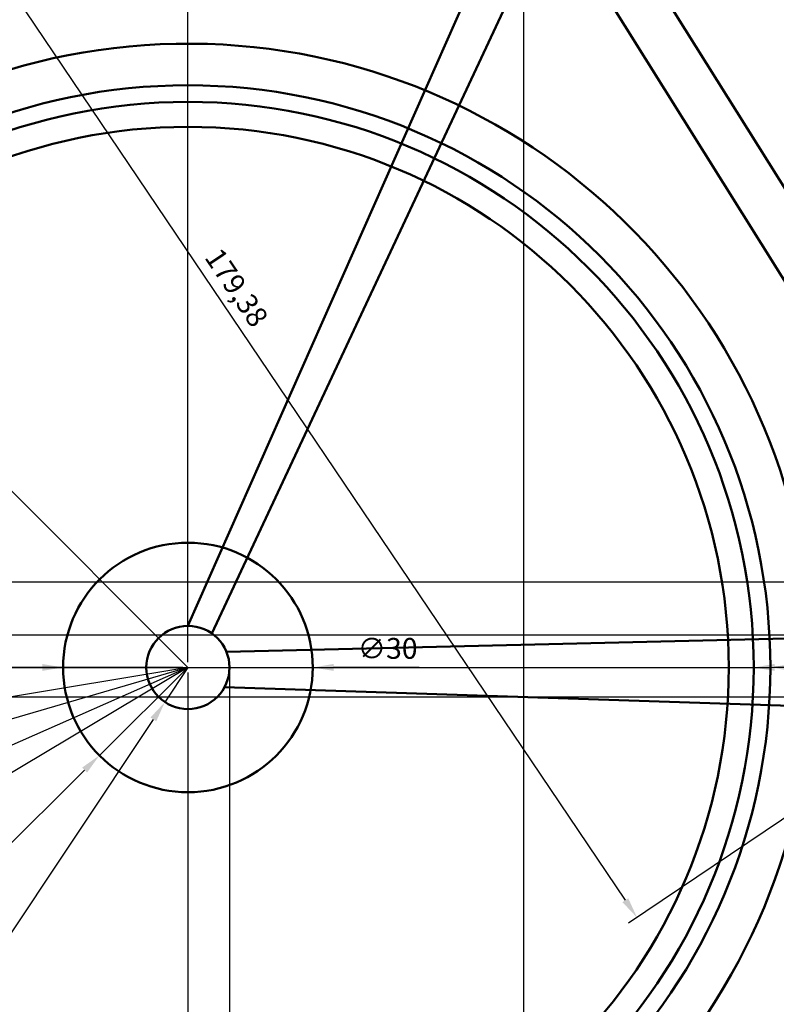
# Model space of a CAD drawing. Units: millimetres. Extents: x 1068 to 1546, y 1743 to 2032.
# Tile 3 of 9: x 1152 to 1243, y 1809 to 1928. Entities that reach past the tile are written whole.
import ezdxf

# ---------------------------------------------------------------- set-up
doc = ezdxf.new("R2010")
doc.units = ezdxf.units.MM
for name, color, linetype, lineweight in [('M-CONS', 8, 'Continuous', 18), ('M-DIMS', 2, 'Continuous', 25), ('M-OUTL', 7, 'Continuous', 50)]:
    doc.layers.add(name, color=color, linetype=linetype, lineweight=lineweight)
doc.styles.get("Standard").update_dxf_attribs({"font": 'arial.ttf'})
doc.dimstyles.new('ISO-25', dxfattribs={"dimtxt": 2.5, "dimasz": 2.5, "dimexe": 1.25, "dimexo": 0.625, "dimtad": 1, "dimtxsty": 'Standard', "dimcen": 2.5, "dimadec": 0, "dimazin": 0, "dimtfac": 1, "dimtmove": 0, "dimatfit": 3, "dimfxl": 1, "dimarcsym": 0})

# ---------------------------------------------------------------- blocks, each defined once
blk = doc.blocks.new('*D5')
at = {"layer": 'Defpoints', "color": 0, "transparency": 16777216}
for p in [(1177.23, 1849.76), (1402.23, 1849.76), (1402.23, 1747.98)]:
    blk.add_point(p, dxfattribs=at)
at = {"layer": 'M-DIMS', "color": 0, "lineweight": -2, "transparency": 16777216}
for p, q in [((1177.23, 1849.14), (1177.23, 1746.73)), ((1402.23, 1849.14), (1402.23, 1746.73)), ((1179.73, 1747.98), (1399.73, 1747.98))]:
    blk.add_line(p, q, dxfattribs=at)
at = {"layer": 'M-DIMS', "color": 0, "transparency": 16777216}
for points in [[(1179.73, 1748.39), (1179.73, 1747.56), (1177.23, 1747.98)], [(1399.73, 1748.39), (1399.73, 1747.56), (1402.23, 1747.98)]]:
    blk.add_solid(points, dxfattribs=at)
at = {"layer": 'M-DIMS', "color": 0, "transparency": 16777216, "insert": (1289.73, 1749.88), "char_height": 2.5, "attachment_point": 5}
blk.add_mtext('225', dxfattribs=at)
blk = doc.blocks.new('*D6')
at = {"layer": 'Defpoints', "color": 0, "transparency": 16777216}
for p in [(1172.23, 1849.76), (1270.79, 1849.76), (1270.79, 1762.16)]:
    blk.add_point(p, dxfattribs=at)
at = {"layer": 'M-DIMS', "color": 0, "lineweight": -2, "transparency": 16777216}
for p, q in [((1172.23, 1849.14), (1172.23, 1760.91)), ((1270.79, 1849.14), (1270.79, 1760.91)), ((1174.73, 1762.16), (1268.29, 1762.16))]:
    blk.add_line(p, q, dxfattribs=at)
at = {"layer": 'M-DIMS', "color": 0, "transparency": 16777216}
for points in [[(1174.73, 1762.57), (1174.73, 1761.74), (1172.23, 1762.16)], [(1268.29, 1762.57), (1268.29, 1761.74), (1270.79, 1762.16)]]:
    blk.add_solid(points, dxfattribs=at)
at = {"layer": 'M-DIMS', "color": 0, "transparency": 16777216, "insert": (1221.51, 1764.28), "char_height": 2.5, "attachment_point": 5}
blk.add_mtext('98,56', dxfattribs=at)
blk = doc.blocks.new('*D12')
at = {"layer": 'Defpoints', "color": 0, "transparency": 16777216}
for p in [(1172.23, 1849.76), (1169.46, 1845.6)]:
    blk.add_point(p, dxfattribs=at)
at = {"layer": 'M-DIMS', "color": 0, "lineweight": -2, "transparency": 16777216}
for p, q in [((1172.23, 1849.76), (1169.46, 1845.6)), ((1115.28, 1764.16), (1168.07, 1843.52))]:
    blk.add_line(p, q, dxfattribs=at)
at = {"layer": 'M-DIMS', "color": 0, "transparency": 16777216}
blk.add_solid([(1167.73, 1843.75), (1168.42, 1843.29), (1169.46, 1845.6)], dxfattribs=at)
at = {"layer": 'M-DIMS', "color": 0, "transparency": 16777216, "insert": (1115.17, 1767.42), "char_height": 2.5, "attachment_point": 5, "rotation": 56.3651}
blk.add_mtext('R5', dxfattribs=at)
blk = doc.blocks.new('*D13')
at = {"layer": 'Defpoints', "color": 0, "transparency": 16777216}
for p in [(1172.23, 1849.76), (1161.59, 1839.19)]:
    blk.add_point(p, dxfattribs=at)
at = {"layer": 'M-DIMS', "color": 0, "lineweight": -2, "transparency": 16777216}
for p, q in [((1172.23, 1849.76), (1161.59, 1839.19)), ((1102.29, 1780.3), (1159.81, 1837.43))]:
    blk.add_line(p, q, dxfattribs=at)
at = {"layer": 'M-DIMS', "color": 0, "transparency": 16777216}
blk.add_solid([(1159.52, 1837.73), (1160.11, 1837.13), (1161.59, 1839.19)], dxfattribs=at)
at = {"layer": 'M-DIMS', "color": 0, "transparency": 16777216, "insert": (1103.52, 1784.2), "char_height": 2.5, "attachment_point": 5, "rotation": 44.8055}
blk.add_mtext('R15', dxfattribs=at)
blk = doc.blocks.new('*D14')
at = {"layer": 'Defpoints', "color": 0, "transparency": 16777216}
for p in [(1172.23, 1849.76), (1116.4, 1816.48)]:
    blk.add_point(p, dxfattribs=at)
at = {"layer": 'M-DIMS', "color": 0, "lineweight": -2, "transparency": 16777216}
for p, q in [((1172.23, 1849.76), (1116.4, 1816.48)), ((1080.65, 1795.17), (1114.25, 1815.2))]:
    blk.add_line(p, q, dxfattribs=at)
at = {"layer": 'M-DIMS', "color": 0, "transparency": 16777216}
blk.add_solid([(1114.03, 1815.56), (1114.46, 1814.84), (1116.4, 1816.48)], dxfattribs=at)
at = {"layer": 'M-DIMS', "color": 0, "transparency": 16777216, "insert": (1082.79, 1798.66), "char_height": 2.5, "attachment_point": 5, "rotation": 30.7992}
blk.add_mtext('R65', dxfattribs=at)
blk = doc.blocks.new('*D15')
at = {"layer": 'Defpoints', "color": 0, "transparency": 16777216}
for p in [(1172.23, 1849.76), (1110.01, 1822.32)]:
    blk.add_point(p, dxfattribs=at)
at = {"layer": 'M-DIMS', "color": 0, "lineweight": -2, "transparency": 16777216}
for p, q in [((1172.23, 1849.76), (1110.01, 1822.32)), ((1084.58, 1811.1), (1107.72, 1821.31))]:
    blk.add_line(p, q, dxfattribs=at)
at = {"layer": 'M-DIMS', "color": 0, "transparency": 16777216}
blk.add_solid([(1107.55, 1821.69), (1107.89, 1820.93), (1110.01, 1822.32)], dxfattribs=at)
at = {"layer": 'M-DIMS', "color": 0, "transparency": 16777216, "insert": (1087.12, 1814.3), "char_height": 2.5, "attachment_point": 5, "rotation": 23.7993}
blk.add_mtext('R68', dxfattribs=at)
blk = doc.blocks.new('*D16')
at = {"layer": 'Defpoints', "color": 0, "transparency": 16777216}
for p in [(1172.23, 1849.76), (1105.05, 1830.07)]:
    blk.add_point(p, dxfattribs=at)
at = {"layer": 'M-DIMS', "color": 0, "lineweight": -2, "transparency": 16777216}
for p, q in [((1172.23, 1849.76), (1105.05, 1830.07)), ((1085.78, 1824.42), (1102.66, 1829.37))]:
    blk.add_line(p, q, dxfattribs=at)
at = {"layer": 'M-DIMS', "color": 0, "transparency": 16777216}
blk.add_solid([(1102.54, 1829.77), (1102.77, 1828.97), (1105.05, 1830.07)], dxfattribs=at)
at = {"layer": 'M-DIMS', "color": 0, "transparency": 16777216, "insert": (1088.71, 1827.26), "char_height": 2.5, "attachment_point": 5, "rotation": 16.3386}
blk.add_mtext('R70', dxfattribs=at)
blk = doc.blocks.new('*D17')
at = {"layer": 'Defpoints', "color": 0, "transparency": 16777216}
for p in [(1172.23, 1849.76), (1098.24, 1837.46)]:
    blk.add_point(p, dxfattribs=at)
at = {"layer": 'M-DIMS', "color": 0, "lineweight": -2, "transparency": 16777216}
for p, q in [((1172.23, 1849.76), (1098.24, 1837.46)), ((1080.67, 1834.54), (1095.78, 1837.05))]:
    blk.add_line(p, q, dxfattribs=at)
at = {"layer": 'M-DIMS', "color": 0, "transparency": 16777216}
blk.add_solid([(1095.71, 1837.46), (1095.85, 1836.64), (1098.24, 1837.46)], dxfattribs=at)
at = {"layer": 'M-DIMS', "color": 0, "transparency": 16777216, "insert": (1083.93, 1837), "char_height": 2.5, "attachment_point": 5, "rotation": 9.4427}
blk.add_mtext('R75', dxfattribs=at)
blk = doc.blocks.new('*D23')
at = {"layer": 'Defpoints', "color": 0, "transparency": 16777216}
for p in [(1170.51, 1998.5), (1125.92, 1968.44), (1270.79, 1849.76)]:
    blk.add_point(p, dxfattribs=at)
at = {"layer": 'M-DIMS', "color": 0, "lineweight": -2, "transparency": 16777216}
for p, q in [((1169.99, 1998.15), (1124.89, 1967.74)), ((1224.8, 1821.77), (1127.32, 1966.36)), ((1270.27, 1849.41), (1225.16, 1819))]:
    blk.add_line(p, q, dxfattribs=at)
at = {"layer": 'M-DIMS', "color": 0, "transparency": 16777216}
for points in [[(1127.67, 1966.6), (1126.98, 1966.13), (1125.92, 1968.44)], [(1225.15, 1822.01), (1224.45, 1821.54), (1226.2, 1819.7)]]:
    blk.add_solid(points, dxfattribs=at)
at = {"layer": 'M-DIMS', "color": 0, "transparency": 16777216, "insert": (1177.82, 1895.26), "char_height": 2.5, "attachment_point": 5, "rotation": 303.9872}
blk.add_mtext('179,38', dxfattribs=at)
blk = doc.blocks.new('*D28')
at = {"layer": 'Defpoints', "color": 0, "transparency": 16777216}
for p in [(1071.98, 1946.21), (1212.68, 1946.21), (1172.23, 1849.76)]:
    blk.add_point(p, dxfattribs=at)
at = {"layer": 'M-DIMS', "color": 0, "lineweight": -2, "transparency": 16777216}
for p, q in [((1212.06, 1946.21), (1070.73, 1946.21)), ((1071.98, 1852.26), (1071.98, 1943.71)), ((1171.6, 1849.76), (1070.73, 1849.76))]:
    blk.add_line(p, q, dxfattribs=at)
at = {"layer": 'M-DIMS', "color": 0, "transparency": 16777216}
for points in [[(1071.57, 1943.71), (1072.4, 1943.71), (1071.98, 1946.21)], [(1071.57, 1852.26), (1072.4, 1852.26), (1071.98, 1849.76)]]:
    blk.add_solid(points, dxfattribs=at)
at = {"layer": 'M-DIMS', "color": 0, "transparency": 16777216, "insert": (1070.08, 1897.98), "char_height": 2.5, "attachment_point": 5, "rotation": 90}
blk.add_mtext('96.44', dxfattribs=at)
blk = doc.blocks.new('*D31')
at = {"layer": 'Defpoints', "color": 0, "transparency": 16777216}
for p in [(1199.17, 2028.2), (1199.17, 1978.98), (1172.23, 1849.76)]:
    blk.add_point(p, dxfattribs=at)
at = {"layer": 'M-DIMS', "color": 0, "lineweight": -2, "transparency": 16777216}
for p, q in [((1172.23, 1850.39), (1172.23, 2029.45)), ((1199.17, 1979.6), (1199.17, 2029.45)), ((1174.73, 2028.2), (1196.67, 2028.2))]:
    blk.add_line(p, q, dxfattribs=at)
at = {"layer": 'M-DIMS', "color": 0, "transparency": 16777216}
for points in [[(1174.73, 2028.61), (1174.73, 2027.78), (1172.23, 2028.2)], [(1196.67, 2028.61), (1196.67, 2027.78), (1199.17, 2028.2)]]:
    blk.add_solid(points, dxfattribs=at)
at = {"layer": 'M-DIMS', "color": 0, "transparency": 16777216, "insert": (1185.7, 2030.1), "char_height": 2.5, "attachment_point": 5}
blk.add_mtext('26.94', dxfattribs=at)
blk = doc.blocks.new('*D45')
at = {"layer": 'Defpoints', "color": 0, "transparency": 16777216}
for p in [(1212.56, 1957.56), (1273.55, 1860.03), (1273.55, 1744.51)]:
    blk.add_point(p, dxfattribs=at)
at = {"layer": 'M-DIMS', "color": 0, "lineweight": -2, "transparency": 16777216}
for p, q in [((1212.56, 1956.94), (1212.56, 1743.26)), ((1273.55, 1859.4), (1273.55, 1743.26)), ((1215.06, 1744.51), (1271.05, 1744.51))]:
    blk.add_line(p, q, dxfattribs=at)
at = {"layer": 'M-DIMS', "color": 0, "transparency": 16777216}
for points in [[(1215.06, 1744.93), (1215.06, 1744.1), (1212.56, 1744.51)], [(1271.05, 1744.93), (1271.05, 1744.1), (1273.55, 1744.51)]]:
    blk.add_solid(points, dxfattribs=at)
at = {"layer": 'M-DIMS', "color": 0, "transparency": 16777216, "insert": (1243.05, 1746.41), "char_height": 2.5, "attachment_point": 5}
blk.add_mtext('60.99', dxfattribs=at)
blk = doc.blocks.new('*D46')
at = {"layer": 'Defpoints', "color": 0, "transparency": 16777216}
for p in [(1212.56, 1957.56), (1071.98, 1860.03), (1273.55, 1860.03)]:
    blk.add_point(p, dxfattribs=at)
at = {"layer": 'M-DIMS', "color": 0, "lineweight": -2, "transparency": 16777216}
for p, q in [((1211.93, 1957.56), (1070.73, 1957.56)), ((1071.98, 1955.06), (1071.98, 1862.53)), ((1272.92, 1860.03), (1070.73, 1860.03))]:
    blk.add_line(p, q, dxfattribs=at)
at = {"layer": 'M-DIMS', "color": 0, "transparency": 16777216}
for points in [[(1071.57, 1955.06), (1072.4, 1955.06), (1071.98, 1957.56)], [(1071.57, 1862.53), (1072.4, 1862.53), (1071.98, 1860.03)]]:
    blk.add_solid(points, dxfattribs=at)
at = {"layer": 'M-DIMS', "color": 0, "transparency": 16777216, "insert": (1070.08, 1908.79), "char_height": 2.5, "attachment_point": 5, "rotation": 90}
blk.add_mtext('97.53', dxfattribs=at)
blk = doc.blocks.new('*D50')
at = {"layer": 'Defpoints', "color": 0, "transparency": 16777216}
for p in [(1261.6, 1853.65), (1071.98, 1846.18), (1262.3, 1846.18)]:
    blk.add_point(p, dxfattribs=at)
at = {"layer": 'M-DIMS', "color": 0, "lineweight": -2, "transparency": 16777216}
for p, q in [((1260.97, 1853.65), (1070.73, 1853.65)), ((1071.98, 1851.15), (1071.98, 1848.68)), ((1261.67, 1846.18), (1070.73, 1846.18)), ((1071.98, 1846.18), (1071.98, 1834.5))]:
    blk.add_line(p, q, dxfattribs=at)
at = {"layer": 'M-DIMS', "color": 0, "transparency": 16777216}
for points in [[(1071.57, 1851.15), (1072.4, 1851.15), (1071.98, 1853.65)], [(1071.57, 1848.68), (1072.4, 1848.68), (1071.98, 1846.18)]]:
    blk.add_solid(points, dxfattribs=at)
at = {"layer": 'M-DIMS', "color": 0, "transparency": 16777216, "insert": (1070.1, 1839.09), "char_height": 2.5, "attachment_point": 5, "rotation": 90}
blk.add_mtext('7.471', dxfattribs=at)
blk = doc.blocks.new('*D57')
at = {"layer": 'Defpoints', "color": 0, "transparency": 16777216}
for p in [(1119.2, 1902.8), (1172.23, 1849.76)]:
    blk.add_point(p, dxfattribs=at)
at = {"layer": 'M-DIMS', "color": 0, "lineweight": -2, "transparency": 16777216}
for p, q in [((1084.82, 1937.18), (1117.43, 1904.57)), ((1172.23, 1849.76), (1119.2, 1902.8))]:
    blk.add_line(p, q, dxfattribs=at)
at = {"layer": 'M-DIMS', "color": 0, "transparency": 16777216}
blk.add_solid([(1117.73, 1904.86), (1117.14, 1904.27), (1119.2, 1902.8)], dxfattribs=at)
at = {"layer": 'M-DIMS', "color": 0, "transparency": 16777216, "insert": (1088.72, 1935.96), "char_height": 2.5, "attachment_point": 5, "rotation": 314.9948}
blk.add_mtext('R75', dxfattribs=at)
blk = doc.blocks.new('*D58')
at = {"layer": 'Defpoints', "color": 0, "transparency": 16777216}
for p in [(1102.23, 1849.76), (1242.23, 1849.76)]:
    blk.add_point(p, dxfattribs=at)
at = {"layer": 'M-DIMS', "color": 0, "lineweight": -2, "transparency": 16777216}
for p, q in [((1099.73, 1849.76), (1097.23, 1849.76)), ((1102.23, 1849.76), (1242.23, 1849.76)), ((1288.97, 1849.76), (1244.73, 1849.76))]:
    blk.add_line(p, q, dxfattribs=at)
at = {"layer": 'M-DIMS', "color": 0, "transparency": 16777216}
for points in [[(1099.73, 1850.18), (1099.73, 1849.35), (1102.23, 1849.76)], [(1244.73, 1850.18), (1244.73, 1849.35), (1242.23, 1849.76)]]:
    blk.add_solid(points, dxfattribs=at)
at = {"layer": 'M-DIMS', "color": 0, "transparency": 16777216, "insert": (1284.23, 1851.73), "char_height": 2.5, "attachment_point": 5, "rotation": 359.9997}
blk.add_mtext('∅140', dxfattribs=at)
blk = doc.blocks.new('*D59')
at = {"layer": 'Defpoints', "color": 0, "transparency": 16777216}
for p in [(1104.23, 1849.76), (1240.23, 1849.76)]:
    blk.add_point(p, dxfattribs=at)
at = {"layer": 'M-DIMS', "color": 0, "lineweight": -2, "transparency": 16777216}
for p, q in [((1101.73, 1849.76), (1099.23, 1849.76)), ((1104.23, 1849.76), (1240.23, 1849.76)), ((1285.77, 1849.76), (1242.73, 1849.76))]:
    blk.add_line(p, q, dxfattribs=at)
at = {"layer": 'M-DIMS', "color": 0, "transparency": 16777216}
for points in [[(1101.73, 1850.18), (1101.73, 1849.35), (1104.23, 1849.76)], [(1242.73, 1850.18), (1242.73, 1849.35), (1240.23, 1849.76)]]:
    blk.add_solid(points, dxfattribs=at)
at = {"layer": 'M-DIMS', "color": 0, "transparency": 16777216, "insert": (1281.03, 1851.73), "char_height": 2.5, "attachment_point": 5, "rotation": 359.9997}
blk.add_mtext('∅136', dxfattribs=at)
blk = doc.blocks.new('*D60')
at = {"layer": 'Defpoints', "color": 0, "transparency": 16777216}
for p in [(1157.23, 1849.76), (1187.23, 1849.76)]:
    blk.add_point(p, dxfattribs=at)
at = {"layer": 'M-DIMS', "color": 0, "lineweight": -2, "transparency": 16777216}
for p, q in [((1154.73, 1849.76), (1152.23, 1849.76)), ((1157.23, 1849.76), (1187.23, 1849.76)), ((1200, 1849.76), (1189.73, 1849.76))]:
    blk.add_line(p, q, dxfattribs=at)
at = {"layer": 'M-DIMS', "color": 0, "transparency": 16777216}
for points in [[(1154.73, 1850.18), (1154.73, 1849.35), (1157.23, 1849.76)], [(1189.73, 1850.18), (1189.73, 1849.35), (1187.23, 1849.76)]]:
    blk.add_solid(points, dxfattribs=at)
at = {"layer": 'M-DIMS', "color": 0, "transparency": 16777216, "insert": (1196.23, 1851.73), "char_height": 2.5, "attachment_point": 5, "rotation": 359.9988}
blk.add_mtext('∅30', dxfattribs=at)

msp = doc.modelspace()

# ---------------------------------------------------------------- linework, layer by layer
at = {"layer": 'M-CONS'}
for q in [(1402.2281, 1849.7623), (1270.787, 1849.7623)]:
    msp.add_line((1172.2281, 1849.7623), q, dxfattribs=at)
at = {"layer": 'M-OUTL'}
for p, q in [((1272.1243, 1862.3034), (1199.166, 1978.9798)), ((1172.2281, 1854.7623), (1212.6811, 1946.2068)), ((1175.1069, 1853.8504), (1215.8973, 1941.0634)), ((1267.1078, 1859.1666), (1215.8973, 1941.0634)), ((1176.8658, 1851.631), (1260.3118, 1853.653)), ((1176.626, 1847.3836), (1260.7126, 1844.644))]:
    msp.add_line(p, q, dxfattribs=at)
for radius in [70, 68, 65, 15, 5]:
    msp.add_circle((1172.2281, 1849.7623), radius, dxfattribs=at)
msp.add_arc((1172.2281, 1849.7623), 75, 2.898254, 355.67622, dxfattribs=at)

# ---------------------------------------------------------------- dimensions: what is measured, and where the dimension line sits
at = {"layer": 'M-DIMS'}
for base, p1, p2, override, picture, middle in [((1199.166, 2028.1976), (1172.2281, 1849.7623), (1199.166, 1978.9798), {"dimdec": 2, "dimlfac": 1, "dimrnd": 0, "dimzin": 0, "dimdsep": 46, "dimlunit": 2}, '*D31', (1185.697, 2030.099)), ((1273.5484, 1744.5123), (1212.5594, 1957.5607), (1273.5484, 1860.0259), {"dimdec": 2, "dimlfac": 1, "dimrnd": 0, "dimzin": 0, "dimdsep": 46, "dimlunit": 2}, '*D45', (1243.0539, 1746.4138)), ((1270.787, 1762.1558), (1172.2281, 1849.7623), (1270.787, 1849.7623), {"dimclrd": 0, "dimclre": 0, "dimclrt": 0}, '*D6', (1221.5076, 1764.2832)), ((1402.2281, 1747.9766), (1177.2281, 1849.7623), (1402.2281, 1849.7623), {"dimclrd": 0, "dimclre": 0, "dimclrt": 0}, '*D5', (1289.7281, 1749.8781))]:
    dim = msp.add_linear_dim(base=base, p1=p1, p2=p2, dimstyle='ISO-25', override=override, dxfattribs=at)
    dim.commit()
    dim.dimension.update_dxf_attribs({"geometry": picture, "text_midpoint": middle})
dim = msp.add_aligned_dim(p1=(1270.787, 1849.7623), p2=(1170.5128, 1998.4966), distance=53.7765, dimstyle='ISO-25', override={"dimclrd": 0, "dimclre": 0, "dimclrt": 0}, dxfattribs=at)
dim.commit()
dim.dimension.update_dxf_attribs({"geometry": '*D23', "text_midpoint": (1177.8244, 1895.2572)})
for base, p1, p2, override, picture, middle in [((1071.9839, 1860.0259), (1212.5594, 1957.5607), (1273.5484, 1860.0259), {"dimdec": 2, "dimlfac": 1, "dimrnd": 0, "dimzin": 0, "dimdsep": 46, "dimlunit": 2}, '*D46', (1070.0816, 1908.7933)), ((1071.9839, 1946.2068), (1172.2281, 1849.7623), (1212.6811, 1946.2068), {"dimdec": 2, "dimlfac": 1, "dimrnd": 0, "dimzin": 0, "dimdsep": 46, "dimlunit": 2}, '*D28', (1070.0825, 1897.9845)), ((1071.9839, 1846.1816), (1261.5989, 1853.653), (1262.2997, 1846.1816), {"dimdec": 3, "dimlfac": 1, "dimrnd": 0, "dimzin": 0, "dimdsep": 46, "dimlunit": 2}, '*D50', (1070.1038, 1839.09))]:
    dim = msp.add_linear_dim(base=base, p1=p1, p2=p2, angle=90, dimstyle='ISO-25', override=override, dxfattribs=at)
    dim.commit()
    dim.dimension.update_dxf_attribs({"geometry": picture, "text_midpoint": middle})
for mpoint, override, picture, middle in [((1119.1999, 1902.8001), {"dimdec": 0, "dimlfac": 1, "dimrnd": 0, "dimzin": 0, "dimdsep": 46, "dimlunit": 2}, '*D57', (1087.383, 1934.6228)), ((1116.3952, 1816.4804), {"dimclrd": 0, "dimclre": 0, "dimclrt": 0}, '*D14', (1083.764, 1797.0289)), ((1098.2444, 1837.4577), {"dimclrd": 0, "dimclre": 0, "dimclrt": 0}, '*D17', (1084.2443, 1835.1292)), ((1110.0105, 1822.322), {"dimclrd": 0, "dimclre": 0, "dimclrt": 0}, '*D15', (1087.8824, 1812.5626)), ((1105.055, 1830.0704), {"dimclrd": 0, "dimclre": 0, "dimclrt": 0}, '*D16', (1089.2466, 1825.4362)), ((1161.5856, 1839.1918), {"dimclrd": 0, "dimclre": 0, "dimclrt": 0}, '*D13', (1104.8597, 1782.8497)), ((1169.4586, 1845.5994), {"dimclrd": 0, "dimclre": 0, "dimclrt": 0}, '*D12', (1116.7499, 1766.3712))]:
    dim = msp.add_radius_dim(center=(1172.2281, 1849.7623), mpoint=mpoint, dimstyle='ISO-25', override=override, dxfattribs=at)
    dim.commit()
    dim.dimension.update_dxf_attribs({"geometry": picture, "text_midpoint": middle, "dimtype": 164})
for p1, p2, picture, middle in [((1102.2281, 1849.7627), (1242.2281, 1849.762), '*D58', (1284.2281, 1849.7618)), ((1104.2281, 1849.7627), (1240.2281, 1849.762), '*D59', (1281.0281, 1849.7618)), ((1157.2281, 1849.7627), (1187.2281, 1849.762), '*D60', (1196.2281, 1849.7618))]:
    dim = msp.add_diameter_dim_2p(p1=p1, p2=p2, dimstyle='ISO-25', override={"dimdec": 0, "dimlfac": 1, "dimrnd": 0, "dimzin": 0, "dimdsep": 46, "dimlunit": 2}, dxfattribs=at)
    dim.commit()
    dim.dimension.update_dxf_attribs({"geometry": picture, "text_midpoint": middle, "dimtype": 163})

doc.saveas('drawing.dxf')
